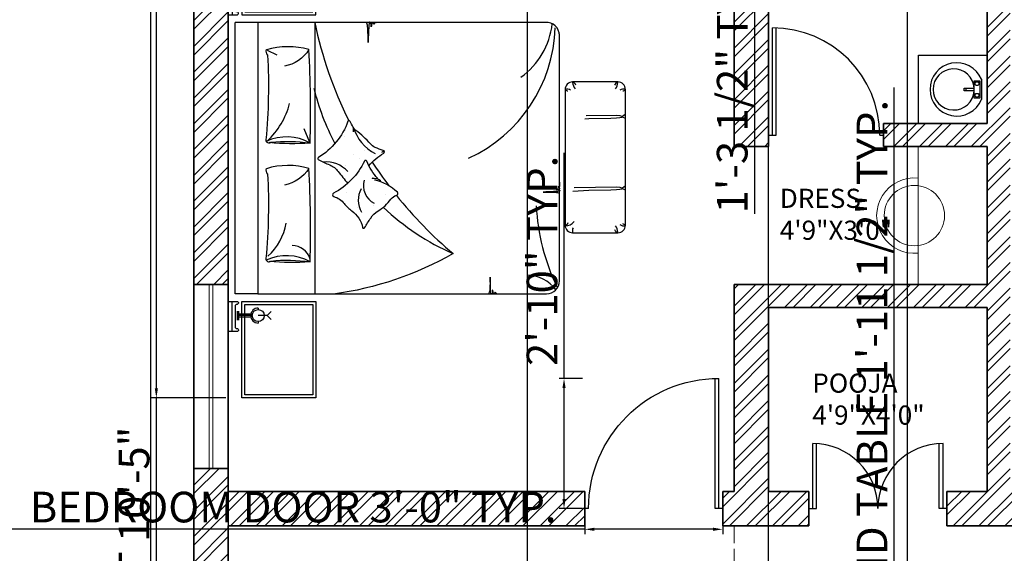
# Model space of a CAD drawing. Units: inches. Extents: x 3595 to 4516, y 2363 to 2965.
# Tile 10 of 12: x 4036 to 4293, y 2686 to 2825. Entities that reach past the tile are written whole.
import ezdxf

# ---------------------------------------------------------------- set-up
doc = ezdxf.new("R2010")
doc.units = ezdxf.units.IN
doc.linetypes.add('ACAD_ISO02W100', pattern=[15, 12, -3])
for name, color, linetype, lineweight in [('A-ANNO-DIMS', 2, 'Continuous', 18), ('A-AREA-IDEN', 7, 'Continuous', 18), ('A-DOOR', 4, 'Continuous', 25), ('A-FLOR-CASE', 9, 'Continuous', 18), ('A-FLOR-FIXT', 8, 'Continuous', 18), ('A-FURN', 43, 'Continuous', 18), ('A-GLAZ', 4, 'Continuous', 18), ('A-WALL', 7, 'Continuous', 35), ('A-WALL-OVHD', 7, 'ACAD_ISO02W100', 18)]:
    doc.layers.add(name, color=color, linetype=linetype, lineweight=lineweight)
doc.layers.add('A-WALL-PATT', color=251, linetype='Continuous', lineweight=13, true_color=0x636466)
for name, color, linetype in [('CEIL', 4, 'Continuous'), ('ELEC', 4, 'Continuous'), ('FUR', 42, 'Continuous'), ('SANTEH', 7, 'Continuous'), ('wood', 26, 'Continuous')]:
    doc.layers.add(name, color=color, linetype=linetype)
doc.styles.get("Standard").update_dxf_attribs({"font": 'arial.ttf'})
doc.dimstyles.new('ISO-25', dxfattribs={"dimtxt": 8, "dimasz": 2.5, "dimexe": 1.25, "dimexo": 0.625, "dimtad": 1, "dimdec": 1, "dimlunit": 3, "dimtxsty": 'Standard', "dimcen": 2.5, "dimadec": 0, "dimazin": 0, "dimtfac": 1, "dimtdec": 1, "dimtmove": 0, "dimatfit": 3, "dimfxl": 1, "dimarcsym": 0})

# ---------------------------------------------------------------- blocks, each defined once
blk = doc.blocks.new('D2')
for p, q in [((1, 0), (1, 28)), ((2, 0), (2, 27.98)), ((0, 0), (2, 0)), ((29, 0), (30, 0))]:
    blk.add_line(p, q)
at = {"ltscale": 0.5}
blk.add_arc((1, 0), 28, 0, 90, dxfattribs=at)
blk = doc.blocks.new('D3')
for p, q in [((1, 0), (1, 17)), ((2, 0), (2, 16.97)), ((34, 0), (34, 16.97)), ((35, 0), (35, 17)), ((0, 0), (2, 0)), ((36, 0), (34, 0))]:
    blk.add_line(p, q)
at = {"ltscale": 0.5}
for centre, start, end in [((1, 0), 0, 90), ((35, 0), 90, 180)]:
    blk.add_arc(centre, 17, start, end, dxfattribs=at)
blk = doc.blocks.new('D1')
for p, q in [((1, 0), (1, 34)), ((2, 0), (2, 33.99)), ((0, 0), (2, 0)), ((35, 0), (36, 0))]:
    blk.add_line(p, q)
at = {"ltscale": 0.5}
blk.add_arc((1, 0), 34, 0, 90, dxfattribs=at)
blk = doc.blocks.new('*D6')
at = {"layer": 'A-ANNO-DIMS', "color": 0, "lineweight": -2, "transparency": 16777216}
for p, q in [((4080.62, 2903.04), (4068.71, 2903.04)), ((4069.96, 2900.54), (4069.96, 2401.54)), ((4080.62, 2399.04), (4068.71, 2399.04))]:
    blk.add_line(p, q, dxfattribs=at)
at = {"layer": 'A-ANNO-DIMS', "color": 0, "transparency": 16777216}
for points in [[(4069.55, 2900.54), (4070.38, 2900.54), (4069.96, 2903.04)], [(4069.55, 2401.54), (4070.38, 2401.54), (4069.96, 2399.04)]]:
    blk.add_solid(points, dxfattribs=at)
at = {"layer": 'Defpoints', "color": 0, "transparency": 16777216}
for p in [(4081.24, 2903.04), (4069.96, 2399.04), (4081.24, 2399.04)]:
    blk.add_point(p, dxfattribs=at)
at = {"layer": 'A-ANNO-DIMS', "color": 0, "transparency": 16777216, "insert": (4065.32, 2651.04), "char_height": 8, "attachment_point": 5, "rotation": 90}
blk.add_mtext("42'", dxfattribs=at)
blk = doc.blocks.new('*X14')
at = {"color": 0}
for p, q in [((3155.9, 8182.9), (3155.9, 8182.9)), ((3147.8, 8143.4), (3147.8, 8143.4)), ((3283, 8049.6), (3283, 8049.6)), ((3209.5, 8023.9), (3209.5, 8023.9)), ((3251.6, 7997), (3251.6, 7997)), ((3154.1, 7950.7), (3154.1, 7950.7))]:
    blk.add_line(p, q, dxfattribs=at)
blk = doc.blocks.new('*X13')
at = {"color": 0}
for p, q in [((3155.9, 8182.9), (3155.9, 8182.9)), ((3139.8, 7939.7), (3139.8, 7939.7))]:
    blk.add_line(p, q, dxfattribs=at)
blk = doc.blocks.new('*X12')
at = {"color": 0}
for p, q in [((3155.9, 8182.9), (3155.9, 8182.9)), ((3139.8, 7939.7), (3139.8, 7939.7))]:
    blk.add_line(p, q, dxfattribs=at)
blk = doc.blocks.new('*X11')
at = {"color": 0}
for p, q in [((3163, 7776.2), (3163, 7776.2)), ((3422.2, 7761.3), (3422.2, 7761.3)), ((3236.2, 7675.7), (3236.2, 7675.7)), ((3244.3, 7698.6), (3244.3, 7698.6)), ((3340.3, 7689.4), (3340.3, 7689.4))]:
    blk.add_line(p, q, dxfattribs=at)
blk = doc.blocks.new('BED1')
for p, q in [((0, -1000), (0, 800)), ((150, 800), (0, 800)), ((150, 800), (150, -1000)), ((2058.7, 800), (150, 800)), ((528, 800), (528, -1000)), ((211.8, 614.9), (277.5, 585.4)), ((2537.2, 404.9), (2237.2, 404.9)), ((2187.2, 354.9), (2187.2, -545.1)), ((2587.2, -545.1), (2587.2, 354.9)), ((2566.3, 178.5), (2565.2, 177.4)), ((2582, 188.1), (2565.4, 174.8)), ((2565.4, 174.8), (2585.7, 165.4)), ((2566.3, -296.8), (2565.2, -297.9)), ((2582, -287.1), (2565.4, -300.5)), ((2565.4, -300.5), (2585.7, -309.9)), ((2237.2, -595.1), (2537.2, -595.1)), ((150, -1000), (0, -1000)), ((150, -1000), (2063.5, -1000))]:
    blk.add_line(p, q)
for points in [[(934, 797.9), (930.9, 797.7), (928.3, 797.4), (926.3, 796.9), (924.9, 796.3), (923.8, 795.6), (923.1, 794.8), (922.7, 793.8), (922.5, 792.7), (922.4, 791.5), (922.5, 790.3), (922.6, 789.2), (922.6, 788.3), (922.6, 787.6), (922.4, 787.3), (922, 787.4), (921.4, 787.9), (920.6, 788.9), (919.5, 790.2), (918.4, 791.6), (917.1, 793.1), (915.9, 794.6), (914.6, 796), (913.3, 797.1), (912.2, 797.9), (911.1, 798.3), (910.1, 798.4), (909.2, 798), (908.3, 797.1), (907.5, 795.8), (906.8, 793.9), (906, 791.4), (905.4, 788.5), (904.8, 785.2), (904.2, 781.7), (903.7, 778.4), (903.2, 775.4), (902.8, 772.9), (902.5, 771.3), (902.3, 770.6), (902.1, 771.2), (902, 772.8), (901.8, 775.2), (901.7, 778.1), (901.5, 781.5), (901.2, 785), (900.8, 788.4), (900.2, 791.5), (899.5, 794.1), (898.6, 796.2), (897.6, 797.9), (896.5, 799.2), (895.3, 800), (894.1, 800.5), (893, 800.7), (891.9, 800.5), (890.9, 800.1), (890, 799), (889.1, 797.1), (888.3, 794), (887.6, 789.3), (886.9, 782.9), (886.2, 774.2), (885.5, 763.1), (884.8, 749.5), (884.2, 734.2), (883.6, 718.3), (883, 702.8), (882.5, 688.8), (882, 677.5), (881.7, 669.8), (881.5, 666.9), (881.3, 669.4), (881.3, 676.7), (881.3, 687.8), (881.2, 701.5), (881.1, 716.8), (880.8, 732.6), (880.2, 748), (879.4, 761.8), (878.3, 773.2), (876.9, 782.2), (875.1, 789.2), (872.9, 794.4), (870.3, 798), (869, 799)], [(2150, -913.5), (2150, 723.2)], [(2327.6, 182.3), (2530, 185.9), (2550.8, 181.9), (2561.7, 179), (2566, 176.7), (2566.9, 174.4), (2566.3, 171.9), (2562, 169.2), (2550.3, 166.5), (2527.7, 163.9), (2490.6, 161.8), (2345.5, 160.2), (2317.8, 158.5)], [(494.7, 3.1), (458.9, 95.3)], [(2149.7, -259.9), (2150, -268.4), (2150.1, -274.1), (2150.1, -278.1), (2150, -281.4), (2149.8, -284), (2149.5, -286.1), (2149.1, -287.8), (2148.7, -289), (2148.1, -289.9), (2147.4, -290.5), (2146.6, -290.8), (2145.6, -291), (2144.6, -291), (2143.6, -291), (2142.7, -290.9), (2141.9, -290.9), (2141.4, -290.9), (2141.1, -291), (2141.2, -291.4), (2141.7, -291.9), (2142.5, -292.6), (2143.5, -293.4), (2144.7, -294.4), (2146, -295.4), (2147.2, -296.5), (2148.4, -297.6), (2149.3, -298.6), (2150, -299.6), (2150.3, -300.5), (2150.4, -301.3), (2150, -302.1), (2149.3, -302.8), (2148.2, -303.5), (2146.6, -304.1), (2144.6, -304.7), (2142.1, -305.2), (2139.3, -305.7), (2136.5, -306.2), (2133.7, -306.6), (2131.2, -307), (2129.2, -307.3), (2127.8, -307.6), (2127.3, -307.8), (2127.7, -308), (2129, -308.1), (2131, -308.2), (2133.5, -308.3), (2136.3, -308.5), (2139.2, -308.7), (2142, -309), (2144.6, -309.5), (2146.8, -310.1), (2148.6, -310.9), (2150, -311.7), (2151, -312.7), (2151.7, -313.6), (2152.1, -314.6), (2152.3, -315.6), (2152.2, -316.5), (2151.8, -317.3), (2150.9, -318.1), (2149.3, -318.8), (2146.7, -319.4), (2142.8, -320), (2137.4, -320.6), (2130.2, -321.2), (2121, -321.8), (2109.7, -322.3), (2096.9, -322.9), (2083.6, -323.4), (2070.7, -323.9), (2059.1, -324.3), (2049.6, -324.7), (2043.2, -325), (2040.8, -325.2), (2042.9, -325.3), (2049, -325.3), (2058.2, -325.3), (2069.6, -325.4), (2082.3, -325.5), (2095.6, -325.8), (2108.4, -326.2), (2119.9, -326.8), (2129.4, -327.8), (2136.9, -329), (2142.7, -330.5), (2147, -332.3), (2150, -334.4), (2150.9, -335.6)], [(2246.5, -294.4), (2530, -289.4), (2550.8, -293.4), (2561.7, -296.3), (2566, -298.6), (2566.9, -300.8), (2566.3, -303.4), (2562, -306.1), (2550.3, -308.8), (2527.7, -311.3), (2490.6, -313.5), (2345.5, -315), (2238.6, -321.8)], [(1733.7, -998.3), (1731.1, -998.1), (1729, -997.8), (1727.4, -997.4), (1726.1, -997), (1725.2, -996.4), (1724.7, -995.7), (1724.3, -994.8), (1724.1, -993.9), (1724.1, -992.9), (1724.1, -991.9), (1724.2, -991), (1724.2, -990.2), (1724.2, -989.7), (1724.1, -989.4), (1723.8, -989.5), (1723.2, -990), (1722.5, -990.8), (1721.7, -991.8), (1720.7, -993), (1719.7, -994.3), (1718.6, -995.5), (1717.5, -996.6), (1716.5, -997.6), (1715.5, -998.3), (1714.6, -998.6), (1713.8, -998.6), (1713, -998.3), (1712.3, -997.6), (1711.7, -996.5), (1711, -994.9), (1710.4, -992.9), (1709.9, -990.4), (1709.4, -987.6), (1708.9, -984.8), (1708.5, -982), (1708.1, -979.5), (1707.8, -977.4), (1707.5, -976.1), (1707.3, -975.5), (1707.1, -976), (1707, -977.3), (1706.9, -979.3), (1706.8, -981.8), (1706.7, -984.6), (1706.4, -987.5), (1706.1, -990.3), (1705.6, -992.9), (1705, -995.1), (1704.2, -996.9), (1703.4, -998.3), (1702.4, -999.3), (1701.5, -1000), (1700.5, -1000.4), (1699.6, -1000.6), (1698.7, -1000.4), (1697.8, -1000.1), (1697, -999.2), (1696.3, -997.6), (1695.7, -995), (1695.1, -991.1), (1694.5, -985.7), (1693.9, -978.5), (1693.3, -969.3), (1692.8, -957.9), (1692.2, -945.2), (1691.7, -931.9), (1691.2, -919), (1690.8, -907.4), (1690.4, -897.9), (1690.1, -891.5), (1689.9, -889.1), (1689.8, -891.2), (1689.8, -897.3), (1689.8, -906.5), (1689.7, -917.9), (1689.6, -930.6), (1689.4, -943.8), (1688.9, -956.6), (1688.3, -968.1), (1687.3, -977.6), (1686.1, -985.2), (1684.6, -991), (1682.8, -995.3), (1680.7, -998.3), (1679.6, -999.2)]]:
    blk.add_lwpolyline(points)
for points in [[(205.5, 619.6, 0.267769), (215.1, 582.4, -0.037739), (204.3, 21.8, 0.684696), (236.7, 5.5, -0.060702), (497.2, 0.1, -0.046649), (225.9, 3.1, -1.318436)], [(489.2, 619.6, 0.144019), (207.6, 617.9, 0.248643)], [(497.2, 0.1, 0.021276), (489.2, 619.6, -0.206383), (326.6, 509.4, 0.237198)], [(211.8, 12.8, 0.143972), (361.6, 262.9, 1.292232)], [(886.4, -150, -0.069098), (985, -66.5, 0.658965), (982.1, -48.7, -0.049789), (927.4, -29, -0.103757), (896.6, -5.4, 0.055725), (800.9, 83.3, -0.11866), (782.7, 104.9, 0.016811), (761.6, 143.9, 0.70791), (748.3, 144, -0.16964), (551.9, -96.6, 0.664036), (554, -110.7, 0.023706), (627, -144.7, -0.134834), (683.2, -188, 0.012748), (746.3, -267.4)], [(969.1, -259.1, 0.263265), (936.3, -236.9, -0.026108), (909.2, -233.2, 0.027613), (945.1, -234.2, -0.089259), (872.7, -120, 0.662242), (857.6, -119.3, -0.162037), (651.8, -332.7, 0.676499), (654, -354.5, -0.160513), (722.9, -401.5, 0.07473), (773.5, -450.3, -0.187721), (845.5, -559.9, 0.70791), (858.8, -561.4, -0.010003), (898.6, -497.3, -0.113819), (947.3, -450.2, 0.099539), (1032.5, -372.4, -0.173425), (1070.9, -346.4, 0.589988), (1076.2, -326.1, 0.137312), (923.9, -245.9, 0.137312)], [(205.5, -168.2, 0.267769), (215.1, -205.4, -0.037739), (204.3, -766, 0.684696), (236.7, -782.3, -0.060702), (497.2, -787.7, -0.046649), (225.9, -784.7, -1.318436)], [(489.2, -168.2, 0.144019), (207.6, -169.9, 0.248643)], [(497.2, -787.7, 0.021276), (489.2, -168.2, -0.206383), (326.6, -278.4, 0.237198)], [(1446, -733.4, -0.095039), (652.8, -1001.7)]]:
    blk.add_lwpolyline(points, format="xyb")
for centre, radius, start, end in [((3208.8, 1363.3), 2739.4, 191.86791, 206.32469), ((1608.1, 842.5), 496.3, 305.19014, 354.02057), ((2062.7, 713.7), 86.5, 0, 93.53765), ((1138.6, 793.9), 983.2, 294.60777, 358.30329), ((2237.2, 354.9), 50, 90, 180), ((2321.1, 409.7), 84.5, 185.61958, 217.13957), ((2227.5, 373.5), 32.8, 17.83305, 72.80048), ((2546.9, 373.5), 32.8, 107.19952, 162.16695), ((2453.3, 409.7), 84.5, 322.86043, 354.38042), ((2537.2, 354.9), 50, 0, 90), ((2098.7, 754.7), 1625, 193.90497, 207.81692), ((2201.9, 323.3), 34.8, 50.8413, 114.9586), ((2212.2, 381.5), 36.5, 226.80948, 258.3841), ((2572.5, 323.3), 34.8, 65.0414, 129.1587), ((2562.2, 381.5), 36.5, 281.6159, 313.19052), ((751.8, 88.7), 34.9, 336.83517, 27.72181), ((684.2, 86), 100.3, 353.675, 10.88198), ((1074.1, 198.8), 306.1, 197.86019, 241.51221), ((341.4, -277.7), 318.5, 60.71255, 115.00895), ((983.7, -79.5), 20.8, 73.79673, 130.45661), ((978.5, -68.6), 14.3, 39.7097, 85.9506), ((602.5, -324), 198.6, 43.20348, 95.05559), ((3208.8, 1363.3), 2739.4, 212.93136, 216.95099), ((981.1, -281.8), 131.1, 164.0372, 243.45361), ((980, -379), 163.4, 152.61037, 209.36102), ((3208.8, 1363.3), 2739.4, 218.63292, 229.94485), ((2098.7, 754.7), 1625, 226.58872, 246.3156), ((3402.5, -342.9), 1408.5, 182.99169, 205.68187), ((2188.1, -476.2), 73, 269.45125, 322.80265), ((-34.4, -471.2), 376.5, 312.01178, 350.96348), ((2178, -513.5), 33, 286.18268, 338.13858), ((2237.2, -545.1), 50, 180, 270), ((2271.1, -580.9), 35.8, 148.90546, 197.55407), ((2546.9, -563.8), 32.8, 197.83305, 252.80048), ((2453.3, -600), 84.5, 5.61958, 37.13957), ((2537.2, -545.1), 50, 270, 0), ((2572.5, -513.6), 34.8, 230.8413, 294.9586), ((2562.2, -571.8), 36.5, 46.80948, 78.3841), ((375.7, -807.4), 128.2, 17.40732, 88.51286), ((341.4, -1065.5), 318.5, 60.71255, 115.00895), ((1929.1, -1126), 250.5, 37.85533, 88.44053), ((2063.5, -913.5), 86.5, 270, 0)]:
    blk.add_arc(centre, radius, start, end)
for name in ['*X13', '*X12', '*X14', '*X11']:
    blk.add_blockref(name, (-2425.3, -8101.4))
blk = doc.blocks.new('APLIQ')
at = {"layer": 'ELEC'}
for p, q in [((0, 0.2), (-0.0261, 0.2261)), ((0, 0.2), (0.0261, 0.2261)), ((0, 0.2), (0, 0.14)), ((-0.05, 0.14), (-0.04, 0.14)), ((0.04, 0.14), (0.05, 0.14)), ((-0.01, 0.09), (-0.01, 0.01)), ((0, 0.09), (0, 0)), ((0.01, 0.09), (0.01, 0.01)), ((-0.03, 0.01), (0.03, 0.01)), ((-0.03, 0), (0.03, 0))]:
    blk.add_line(p, q, dxfattribs=at)
blk.add_circle((0, 0.14), 0.04, dxfattribs=at)
blk.add_arc((0, 0.14), 0.05, 180, 0, dxfattribs=at)
blk = doc.blocks.new('A$C68AE1801')
at = {"layer": 'FUR'}
for points in [[(2.5416, 3.18), (2.5416, 2.54), (2.0516, 2.54), (2.0516, 3.18)], [(2.5216, 3.16), (2.5216, 2.56), (2.0716, 2.56), (2.0716, 3.16)], [(2.5416, 0), (2.5416, 0.64), (2.0516, 0.64), (2.0516, 0)], [(2.5216, 0.02), (2.5216, 0.62), (2.0716, 0.62), (2.0716, 0.02)]]:
    blk.add_lwpolyline(points, close=True, dxfattribs=at)
at = {"layer": 'wood'}
for p, q in [((2.6057, 2.74), (2.6057, 2.54)), ((2.6057, 0.44), (2.6057, 0.64))]:
    blk.add_line(p, q, dxfattribs=at)
for points in [[(2.5657, 2.728), (2.5657, 2.732, -0.414214), (2.5737, 2.74), (2.6321, 2.74), (2.6321, 2.54), (2.5737, 2.54, -0.414214), (2.5657, 2.548), (2.5657, 2.552, -0.414214), (2.5737, 2.56), (2.5777, 2.56, 0.414214), (2.5857, 2.568), (2.5857, 2.712, 0.414214), (2.5777, 2.72), (2.5737, 2.72, -0.414214)], [(2.5657, 0.452), (2.5657, 0.448, 0.414214), (2.5737, 0.44), (2.6321, 0.44), (2.6321, 0.64), (2.5737, 0.64, 0.414214), (2.5657, 0.632), (2.5657, 0.628, 0.414214), (2.5737, 0.62), (2.5777, 0.62, -0.414214), (2.5857, 0.612), (2.5857, 0.468, -0.414214), (2.5777, 0.46), (2.5737, 0.46, 0.414214)]]:
    blk.add_lwpolyline(points, format="xyb", close=True, dxfattribs=at)
at = {"layer": 'CEIL', "rotation": 90}
blk.add_blockref('APLIQ', (2.5736, 2.634), dxfattribs=at)
at = {"layer": 'CEIL', "xscale": -1, "rotation": 90}
blk.add_blockref('APLIQ', (2.5736, 0.546), dxfattribs=at)
at = {"layer": 'FUR', "xscale": 0.001, "yscale": 0.001, "zscale": 0.001, "rotation": 180}
blk.add_blockref('BED1', (2.5872, 1.49), dxfattribs=at)
blk = doc.blocks.new('AP2041')
blk.add_lwpolyline([(198.4, 175), (248.7, 175, 1.105542), (-248.7, 175), (-198.4, 175)], format="xyb")
blk.add_circle((0, 200), 200)
blk = doc.blocks.new('r11')
at = {"layer": 'SANTEH', "ltscale": 5}
for p, q in [((0, 0), (600, 0)), ((0, -600), (0, 0)), ((600, 0), (600, -600)), ((210.5, -50), (389.5, -50)), ((210.5, -50), (210.5, -50)), ((223.8, -63.2), (376.2, -63.2)), ((223.8, -113.2), (223.8, -63.2)), ((232.7, -78.7), (249.2, -69.1)), ((232.7, -97.7), (232.7, -78.7)), ((249.2, -69.1), (265.7, -78.7)), ((265.7, -78.7), (265.7, -97.7)), ((334.3, -78.7), (350.8, -69.1)), ((334.3, -97.7), (334.3, -78.7)), ((350.8, -69.1), (367.3, -78.7)), ((367.3, -78.7), (367.3, -97.7)), ((376.2, -63.2), (376.2, -113.2)), ((376.2, -113.2), (223.8, -113.2)), ((249.2, -107.2), (232.7, -97.7)), ((265.7, -97.7), (249.2, -107.2)), ((288, -201.6), (288, -113.2)), ((312, -113.2), (312, -201.6)), ((350.8, -107.2), (334.3, -97.7)), ((367.3, -97.7), (350.8, -107.2)), ((312, -184.3), (288, -184.3)), ((312, -201.6), (288, -201.6)), ((600, -600), (0, -600))]:
    blk.add_line(p, q, dxfattribs=at)
for centre, radius, start, end in [((300, -266.2), 234, 112.50001, 67.49999), ((300, -293), 180.2, 93.8183, 86.1817)]:
    blk.add_arc(centre, radius, start, end, dxfattribs=at)
blk = doc.blocks.new('WIN-GLAZING-48IN')
for p, q in [((0, 1), (48, 1)), ((0, 0), (48, 0))]:
    blk.add_line(p, q)
blk = doc.blocks.new('*D115')
at = {"layer": 'A-ANNO-DIMS', "color": 0, "lineweight": -2, "transparency": 16777216}
for p, q in [((4183.24, 2696.92), (4183.24, 2690.89)), ((4219.24, 2696.92), (4219.24, 2690.89)), ((4183.24, 2692.14), (4033.6, 2692.14)), ((4216.74, 2692.14), (4185.74, 2692.14))]:
    blk.add_line(p, q, dxfattribs=at)
at = {"layer": 'A-ANNO-DIMS', "color": 0, "transparency": 16777216}
for points in [[(4185.74, 2692.56), (4185.74, 2691.73), (4183.24, 2692.14)], [(4216.74, 2692.56), (4216.74, 2691.73), (4219.24, 2692.14)]]:
    blk.add_solid(points, dxfattribs=at)
at = {"layer": 'Defpoints', "color": 0, "transparency": 16777216}
for p in [(4183.24, 2697.54), (4219.24, 2697.54), (4183.24, 2692.14)]:
    blk.add_point(p, dxfattribs=at)
at = {"layer": 'A-ANNO-DIMS', "color": 0, "transparency": 16777216, "insert": (4107.17, 2696.91), "char_height": 8, "attachment_point": 5}
blk.add_mtext('BEDROOM DOOR 3\'-0" TYP.', dxfattribs=at)
blk = doc.blocks.new('*D116')
at = {"layer": 'A-ANNO-DIMS', "color": 0, "lineweight": -2, "transparency": 16777216}
for p, q in [((4177.84, 2731.54), (4177.84, 2790.41)), ((4182.62, 2731.54), (4176.59, 2731.54)), ((4177.84, 2700.04), (4177.84, 2729.04)), ((4182.62, 2697.54), (4176.59, 2697.54))]:
    blk.add_line(p, q, dxfattribs=at)
at = {"layer": 'A-ANNO-DIMS', "color": 0, "transparency": 16777216}
for points in [[(4177.43, 2729.04), (4178.26, 2729.04), (4177.84, 2731.54)], [(4177.43, 2700.04), (4178.26, 2700.04), (4177.84, 2697.54)]]:
    blk.add_solid(points, dxfattribs=at)
at = {"layer": 'Defpoints', "color": 0, "transparency": 16777216}
for p in [(4177.84, 2731.54), (4183.24, 2731.54), (4183.24, 2697.54)]:
    blk.add_point(p, dxfattribs=at)
at = {"layer": 'A-ANNO-DIMS', "color": 0, "transparency": 16777216, "insert": (4173.13, 2762.23), "char_height": 8, "attachment_point": 5, "rotation": 90}
blk.add_mtext('2\'-10" TYP.', dxfattribs=at)
blk = doc.blocks.new('*D119')
at = {"layer": 'A-ANNO-DIMS', "color": 0, "lineweight": -2, "transparency": 16777216}
for p, q in [((4089.62, 2851.64), (4070.21, 2851.64)), ((4071.46, 2849.14), (4071.46, 2728.95)), ((4089.62, 2726.45), (4070.21, 2726.45)), ((4071.46, 2726.45), (4071.46, 2590.66))]:
    blk.add_line(p, q, dxfattribs=at)
at = {"layer": 'A-ANNO-DIMS', "color": 0, "transparency": 16777216}
for points in [[(4071.05, 2849.14), (4071.88, 2849.14), (4071.46, 2851.64)], [(4071.05, 2728.95), (4071.88, 2728.95), (4071.46, 2726.45)]]:
    blk.add_solid(points, dxfattribs=at)
at = {"layer": 'Defpoints', "color": 0, "transparency": 16777216}
for p in [(4090.24, 2851.64), (4071.46, 2726.45), (4090.24, 2726.45)]:
    blk.add_point(p, dxfattribs=at)
at = {"layer": 'A-ANNO-DIMS', "color": 0, "transparency": 16777216, "insert": (4066.7, 2657.3), "char_height": 8, "attachment_point": 5, "rotation": 90}
blk.add_mtext('PRIMARY BED SET 10\'-5"', dxfattribs=at)
blk = doc.blocks.new('*D132')
at = {"layer": 'A-ANNO-DIMS', "color": 0, "lineweight": -2, "transparency": 16777216}
for p, q in [((4230.62, 2860.28), (4226.27, 2860.28)), ((4227.52, 2857.78), (4227.52, 2847.39)), ((4230.62, 2844.89), (4226.27, 2844.89)), ((4227.52, 2844.89), (4227.52, 2774.49))]:
    blk.add_line(p, q, dxfattribs=at)
at = {"layer": 'A-ANNO-DIMS', "color": 0, "transparency": 16777216}
for points in [[(4227.11, 2857.78), (4227.94, 2857.78), (4227.52, 2860.28)], [(4227.11, 2847.39), (4227.94, 2847.39), (4227.52, 2844.89)]]:
    blk.add_solid(points, dxfattribs=at)
at = {"layer": 'Defpoints', "color": 0, "transparency": 16777216}
for p in [(4231.24, 2860.28), (4227.52, 2844.89), (4231.24, 2844.89)]:
    blk.add_point(p, dxfattribs=at)
at = {"layer": 'A-ANNO-DIMS', "color": 0, "transparency": 16777216, "insert": (4222.76, 2808.44), "char_height": 8, "attachment_point": 5, "rotation": 90}
blk.add_mtext('1\'-3 1/2" TYP.', dxfattribs=at)
blk = doc.blocks.new('*D141')
at = {"layer": 'A-ANNO-DIMS', "color": 0, "lineweight": -2, "transparency": 16777216}
for p, q in [((4264, 2665.33), (4264, 2807.49)), ((4266.92, 2665.33), (4262.75, 2665.33)), ((4264, 2644.21), (4264, 2662.83)), ((4266.92, 2641.71), (4262.75, 2641.71))]:
    blk.add_line(p, q, dxfattribs=at)
at = {"layer": 'A-ANNO-DIMS', "color": 0, "transparency": 16777216}
for points in [[(4263.59, 2662.83), (4264.42, 2662.83), (4264, 2665.33)], [(4263.59, 2644.21), (4264.42, 2644.21), (4264, 2641.71)]]:
    blk.add_solid(points, dxfattribs=at)
at = {"layer": 'Defpoints', "color": 0, "transparency": 16777216}
for p in [(4264, 2665.33), (4267.55, 2665.33), (4267.55, 2641.71)]:
    blk.add_point(p, dxfattribs=at)
at = {"layer": 'A-ANNO-DIMS', "color": 0, "transparency": 16777216, "insert": (4259.24, 2737.66), "char_height": 8, "attachment_point": 5, "rotation": 90}
blk.add_mtext('END TABLE 1\'-11 1/2" TYP.', dxfattribs=at)
blk = doc.blocks.new('*D163')
at = {"layer": 'A-ANNO-DIMS', "color": 0, "lineweight": -2, "transparency": 16777216}
for p, q in [((4267.47, 2626.41), (4267.47, 2932.84)), ((4269.97, 2931.59), (4292.53, 2931.59)), ((4295.03, 2624.44), (4295.03, 2932.84)), ((4295.03, 2931.59), (4338.82, 2931.59))]:
    blk.add_line(p, q, dxfattribs=at)
at = {"layer": 'A-ANNO-DIMS', "color": 0, "transparency": 16777216}
for points in [[(4269.97, 2932.01), (4269.97, 2931.18), (4267.47, 2931.59)], [(4292.53, 2932.01), (4292.53, 2931.18), (4295.03, 2931.59)]]:
    blk.add_solid(points, dxfattribs=at)
at = {"layer": 'Defpoints', "color": 0, "transparency": 16777216}
for p in [(4295.03, 2931.59), (4267.47, 2625.78), (4295.03, 2623.82)]:
    blk.add_point(p, dxfattribs=at)
at = {"layer": 'A-ANNO-DIMS', "color": 0, "transparency": 16777216, "insert": (4318.18, 2936.36), "char_height": 8, "attachment_point": 5}
blk.add_mtext('2\'-3 1/2"', dxfattribs=at)
blk = doc.blocks.new('*D167')
at = {"layer": 'A-ANNO-DIMS', "color": 0, "lineweight": -2, "transparency": 16777216}
for p, q in [((4231.24, 2606.67), (4231.24, 2932.84)), ((4233.74, 2931.59), (4264.97, 2931.59)), ((4267.47, 2626.41), (4267.47, 2932.84))]:
    blk.add_line(p, q, dxfattribs=at)
at = {"layer": 'A-ANNO-DIMS', "color": 0, "transparency": 16777216}
for points in [[(4233.74, 2932.01), (4233.74, 2931.18), (4231.24, 2931.59)], [(4264.97, 2932.01), (4264.97, 2931.18), (4267.47, 2931.59)]]:
    blk.add_solid(points, dxfattribs=at)
at = {"layer": 'Defpoints', "color": 0, "transparency": 16777216}
for p in [(4267.47, 2931.59), (4267.47, 2625.78), (4231.24, 2606.04)]:
    blk.add_point(p, dxfattribs=at)
at = {"layer": 'A-ANNO-DIMS', "color": 0, "transparency": 16777216, "insert": (4249.36, 2936.31), "char_height": 8, "attachment_point": 5}
blk.add_mtext('3\'-0"', dxfattribs=at)
blk = doc.blocks.new('*D170')
at = {"layer": 'A-ANNO-DIMS', "color": 0, "lineweight": -2, "transparency": 16777216}
for p, q in [((4090.24, 2875.42), (4090.24, 2369.24)), ((4168.24, 2875.42), (4168.24, 2369.24)), ((4092.74, 2370.49), (4165.74, 2370.49))]:
    blk.add_line(p, q, dxfattribs=at)
at = {"layer": 'A-ANNO-DIMS', "color": 0, "transparency": 16777216}
for points in [[(4092.74, 2370.91), (4092.74, 2370.08), (4090.24, 2370.49)], [(4165.74, 2370.91), (4165.74, 2370.08), (4168.24, 2370.49)]]:
    blk.add_solid(points, dxfattribs=at)
at = {"layer": 'Defpoints', "color": 0, "transparency": 16777216}
for p in [(4090.24, 2876.04), (4168.24, 2876.04), (4168.24, 2370.49)]:
    blk.add_point(p, dxfattribs=at)
at = {"layer": 'A-ANNO-DIMS', "color": 0, "transparency": 16777216, "insert": (4129.24, 2375.2), "char_height": 8, "attachment_point": 5}
blk.add_mtext('6\'-6"', dxfattribs=at)

msp = doc.modelspace()

# ---------------------------------------------------------------- hatches: boundary and pattern name
at = {"layer": 'A-WALL-PATT'}
h = msp.add_hatch(dxfattribs=at)
h.set_pattern_fill('ANSI32', color=256, scale=0.5)
h.set_pattern_definition([(45, (441.351, 0), (-3.367596, 3.367596), []), (45, (443.596, 0), (-3.367596, 3.367596), [])])
h.paths.add_polyline_path([(4081.24, 2756.04), (4090.24, 2756.04), (4090.24, 2894.04), (4168.24, 2894.04), (4168.24, 2903.04), (4081.24, 2903.04)])
h.paths.add_polyline_path([(4216.24, 2903.04), (4216.24, 2894.04), (4222.24, 2894.04), (4222.24, 2792.04), (4231.24, 2792.04), (4231.24, 2894.04), (4241.74, 2894.04), (4241.74, 2903.04)])
h.paths.add_polyline_path([(4324.24, 2894.04), (4324.24, 2903.04), (4277.74, 2903.04), (4277.74, 2894.04), (4288.24, 2894.04), (4288.24, 2798.04), (4261.24, 2798.04), (4261.24, 2792.04), (4288.24, 2792.04), (4288.24, 2756.04), (4222.24, 2756.04), (4222.24, 2702.04), (4219.24, 2702.04), (4219.24, 2693.04), (4241.74, 2693.04), (4241.74, 2702.04), (4231.24, 2702.04), (4231.24, 2750.04), (4288.24, 2750.04), (4288.24, 2702.04), (4277.74, 2702.04), (4277.74, 2693.04), (4393.24, 2693.04), (4393.24, 2702.04), (4294.24, 2702.04), (4294.24, 2840.04), (4396.24, 2840.04), (4396.24, 2846.04), (4294.24, 2846.04), (4294.24, 2894.04)])
h.paths.add_polyline_path([(4390.24, 2894.04), (4390.24, 2876.04), (4396.24, 2876.04), (4396.24, 2894.04), (4432.24, 2894.04), (4432.24, 2795.04), (4441.24, 2795.04), (4441.24, 2903.04), (4360.24, 2903.04), (4360.24, 2894.04)])
h.paths.add_polyline_path([(4090.24, 2693.04), (4183.24, 2693.04), (4183.24, 2702.04), (4090.24, 2702.04), (4090.24, 2708.04), (4081.24, 2708.04), (4081.24, 2673.54), (4090.24, 2673.54)])
h.paths.add_polyline_path([(4090.24, 2600.04), (4183.24, 2600.04), (4183.24, 2606.04), (4090.24, 2606.04), (4090.24, 2625.54), (4081.24, 2625.54), (4081.24, 2561.04), (4090.24, 2561.04)])
h.paths.add_polyline_path([(4081.24, 2399.04), (4231.24, 2399.04), (4231.24, 2405.04), (4090.24, 2405.04), (4090.24, 2477.04), (4180.24, 2477.04), (4180.24, 2486.04), (4090.24, 2486.04), (4090.24, 2525.04), (4081.24, 2525.04)])
h.paths.add_polyline_path([(4231.24, 2486.04), (4231.24, 2606.04), (4219.24, 2606.04), (4219.24, 2600.04), (4222.24, 2600.04), (4222.24, 2486.04), (4216.24, 2486.04), (4216.24, 2477.04), (4273.24, 2477.04), (4273.24, 2486.04)])
h.paths.add_polyline_path([(4339.24, 2486.04), (4339.24, 2477.04), (4381.24, 2477.04), (4381.24, 2486.04)])
h.paths.add_polyline_path([(4432.24, 2486.04), (4429.24, 2486.04), (4429.24, 2477.04), (4441.24, 2477.04), (4441.24, 2511.54), (4432.24, 2511.54)])
h.paths.add_polyline_path([(4432.24, 2571.54), (4441.24, 2571.54), (4441.24, 2607.54), (4432.24, 2607.54)])
h.paths.add_polyline_path([(4441.24, 2747.04), (4432.24, 2747.04), (4432.24, 2702.04), (4429.24, 2702.04), (4429.24, 2693.04), (4432.24, 2693.04), (4432.24, 2667.54), (4441.24, 2667.54)])

# ---------------------------------------------------------------- linework, layer by layer
at = {"layer": 'A-FLOR-CASE'}
msp.add_line((4270.24, 2756.04), (4270.24, 2792.04), dxfattribs=at)
at = {"layer": 'A-WALL'}
for p, q in [((4090.24, 2702.04), (4090.24, 2894.04)), ((4222.24, 2792.04), (4222.24, 2894.04)), ((4231.24, 2792.04), (4231.24, 2894.04)), ((4288.24, 2798.04), (4288.24, 2894.04)), ((4261.24, 2792.04), (4261.24, 2798.04)), ((4261.24, 2798.04), (4288.24, 2798.04)), ((4222.24, 2792.04), (4231.24, 2792.04)), ((4261.24, 2792.04), (4288.24, 2792.04)), ((4288.24, 2756.04), (4288.24, 2792.04)), ((4081.24, 2756.04), (4090.24, 2756.04)), ((4222.24, 2702.04), (4222.24, 2756.04)), ((4222.24, 2756.04), (4288.24, 2756.04)), ((4231.24, 2702.04), (4231.24, 2750.04)), ((4231.24, 2750.04), (4288.24, 2750.04)), ((4288.24, 2702.04), (4288.24, 2750.04)), ((4081.24, 2708.04), (4090.24, 2708.04)), ((4090.24, 2702.04), (4183.24, 2702.04)), ((4183.24, 2693.04), (4183.24, 2702.04)), ((4219.24, 2702.04), (4222.24, 2702.04)), ((4219.24, 2693.04), (4219.24, 2702.04)), ((4231.24, 2702.04), (4241.74, 2702.04)), ((4241.74, 2702.04), (4241.74, 2693.04)), ((4277.74, 2702.04), (4288.24, 2702.04)), ((4277.74, 2702.04), (4277.74, 2693.04)), ((4090.24, 2693.04), (4183.24, 2693.04)), ((4090.24, 2606.04), (4090.24, 2693.04)), ((4219.24, 2693.04), (4241.74, 2693.04)), ((4277.74, 2693.04), (4393.24, 2693.04))]:
    msp.add_line(p, q, dxfattribs=at)
msp.add_lwpolyline([(4231.24, 2399.04), (4081.24, 2399.04), (4081.24, 2903.04), (4441.24, 2903.04), (4441.24, 2477.04)], dxfattribs=at)
at = {"layer": 'A-WALL-OVHD', "ltscale": 0.5}
for p, q in [((4222.24, 2606.04), (4222.24, 2693.04)), ((4231.24, 2606.04), (4231.24, 2693.04))]:
    msp.add_line(p, q, dxfattribs=at)

# ---------------------------------------------------------------- block references
at = {"layer": 'A-DOOR'}
for name, p in [('D2', (4231.24, 2795.04)), ('D3', (4241.74, 2697.54))]:
    msp.add_blockref(name, p, dxfattribs=at)
at = {"layer": 'A-DOOR', "xscale": -1}
msp.add_blockref('D1', (4219.24, 2697.54), dxfattribs=at)
at = {"layer": 'A-FLOR-FIXT', "xscale": 0.0297800069284724, "yscale": 0.0297800069284724, "zscale": 0.0297800069284724, "rotation": 270}
msp.add_blockref('r11', (4288.24, 2815.91), dxfattribs=at)
at = {"layer": 'A-FURN'}
for name, p, xscale, yscale, zscale, rotation in [('A$C68AE1801', (4193.87, 2851.64), 39.3701, 39.3701, 39.3701, 180), ('AP2041', (4277.13, 2774.04), 0.0393701, 0.0393701, 0.0393701, 90)]:
    msp.add_blockref(name, p, dxfattribs=dict(at, xscale=xscale, yscale=yscale, zscale=zscale, rotation=rotation))
at = {"layer": 'A-GLAZ', "rotation": 270}
msp.add_blockref('WIN-GLAZING-48IN', (4085.24, 2756.04), dxfattribs=at)

# ---------------------------------------------------------------- texts
at = {"layer": 'A-AREA-IDEN', "char_height": 5, "attachment_point": 1}
for s, insert in [('{\\fTimes New Roman|b0|i0|c0|p18;DRESS\\P4\'9"X3\'0"}', (4234.15, 2781.05)), ('{\\fTimes New Roman|b0|i0|c0|p18;POOJA\\P4\'9"X4\'0"}', (4242.62, 2732.8))]:
    msp.add_mtext_dynamic_manual_height_columns(s, width=67.3508, gutter_width=12.5, heights=[0], dxfattribs=dict(at, insert=insert))

# ---------------------------------------------------------------- dimensions: what is measured, and where the dimension line sits
at = {"layer": 'A-ANNO-DIMS'}
for base, p1, p2, picture, middle in [((4295.03, 2931.59), (4267.47, 2625.78), (4295.03, 2623.82), '*D163', (4318.18, 2936.36)), ((4267.47, 2931.59), (4231.24, 2606.04), (4267.47, 2625.78), '*D167', (4249.36, 2936.31)), ((4168.24, 2370.49), (4090.24, 2876.04), (4168.24, 2876.04), '*D170', (4129.24, 2375.2))]:
    dim = msp.add_linear_dim(base=base, p1=p1, p2=p2, dimstyle='ISO-25', override={"dimdec": 1, "dimlfac": 1, "dimrnd": 0, "dimzin": 1, "dimdsep": 46, "dimlunit": 4, "dimfrac": 2}, dxfattribs=at)
    dim.commit()
    dim.dimension.update_dxf_attribs({"geometry": picture, "text_midpoint": middle})
dim = msp.add_linear_dim(base=(4069.96, 2399.04), p1=(4081.24, 2903.04), p2=(4081.24, 2399.04), angle=90, dimstyle='ISO-25', override={"dimclrd": 0, "dimclre": 0, "dimclrt": 0}, dxfattribs=at)
dim.commit()
dim.dimension.update_dxf_attribs({"geometry": '*D6', "text_midpoint": (4065.32, 2651.04)})
for base, p1, p2, angle, text, picture, middle in [((4227.52, 2844.89), (4231.24, 2860.28), (4231.24, 2844.89), 270, '<> TYP.', '*D132', (4222.76, 2808.44)), ((4071.46, 2726.45), (4090.24, 2851.64), (4090.24, 2726.45), 270, 'PRIMARY BED SET <>', '*D119', (4066.7, 2657.3)), ((4264, 2665.33), (4267.55, 2641.71), (4267.55, 2665.33), 90, 'END TABLE <> TYP.', '*D141', (4259.24, 2737.66)), ((4177.84, 2731.54), (4183.24, 2697.54), (4183.24, 2731.54), 90, '<> TYP.', '*D116', (4173.13, 2762.23)), ((4183.24, 2692.14), (4219.24, 2697.54), (4183.24, 2697.54), 180, 'BEDROOM DOOR <> TYP.', '*D115', (4107.17, 2696.91))]:
    dim = msp.add_linear_dim(base=base, p1=p1, p2=p2, angle=angle, text=text, dimstyle='ISO-25', override={"dimdec": 1, "dimlfac": 1, "dimrnd": 0, "dimzin": 1, "dimdsep": 46, "dimlunit": 4, "dimfrac": 2}, dxfattribs=at)
    dim.commit()
    dim.dimension.update_dxf_attribs({"geometry": picture, "text_midpoint": middle})

doc.saveas('drawing.dxf')
